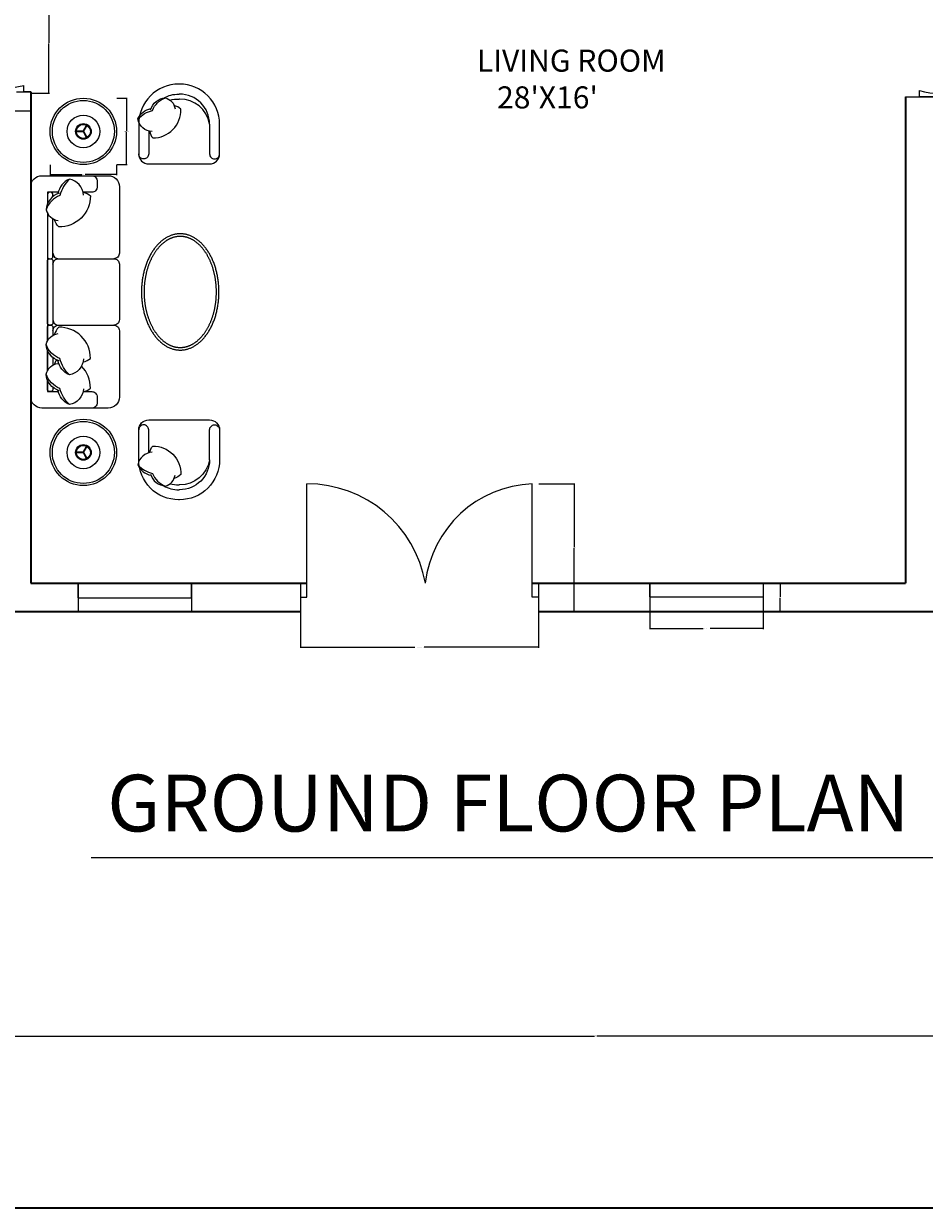
# Model space of a CAD drawing. Units: inches. Extents: x 2185 to 4426, y 1138 to 3073.
# Tile 2 of 14: x 2548 to 2834, y 1138 to 1514. Entities that reach past the tile are written whole.
import ezdxf

# ---------------------------------------------------------------- set-up
doc = ezdxf.new("R2010")
doc.units = ezdxf.units.IN
for name, color, linetype, lineweight in [('A-ANNO-DIMS', 2, 'Continuous', 18), ('A-ANNO-TITL', 7, 'Continuous', 25), ('A-ANNO-TTLB', 7, 'Continuous', 35), ('A-AREA-IDEN', 7, 'Continuous', 18), ('A-DOOR', 3, 'Continuous', 18), ('A-FURN', 8, 'Continuous', 18), ('A-GLAZ', 4, 'Continuous', 18), ('A-WALL', 7, 'Continuous', 35)]:
    doc.layers.add(name, color=color, linetype=linetype, lineweight=lineweight)
doc.styles.get("Standard").update_dxf_attribs({"font": 'arial.ttf'})
doc.dimstyles.get("Standard").update_dxf_attribs({"dimtxt": 0.18, "dimasz": 0.18, "dimexe": 0.18, "dimexo": 0.0625, "dimgap": 0.09, "dimtad": 0, "dimtih": 1, "dimtoh": 1, "dimdec": 4, "dimzin": 0, "dimdsep": 46, "dimtxsty": 'Standard', "dimcen": 0.09, "dimadec": 0, "dimazin": 0, "dimtfac": 1, "dimtdec": 4, "dimtofl": 0, "dimtmove": 0, "dimatfit": 3, "dimfxl": 1, "dimtolj": 1, "dimtzin": 0, "dimarcsym": 0})

# ---------------------------------------------------------------- blocks, each defined once
blk = doc.blocks.new('LIVING-TABLE-LAMP')
at = {"ltscale": 0.03}
for p, q in [((10.44, 10.59), (11.68, 12.74)), ((10.63, 10.48), (11.87, 12.63)), ((10.54, 10.65), (8.06, 10.65)), ((10.54, 10.43), (8.06, 10.43)), ((10.44, 10.48), (11.68, 8.34)), ((10.63, 10.59), (11.87, 8.45))]:
    blk.add_line(p, q, dxfattribs=at)
for radius in [10.54, 5.18, 2.48, 2.22]:
    blk.add_circle((10.54, 10.54), radius, dxfattribs=at)
blk.add_circle((10.54, 10.54), 9.84)
blk = doc.blocks.new('DOOR-SGL-36-BED-SW')
for p, q in [((38.25, 31.13), (33.75, 31.13)), ((33.75, 31.13), (36, 31.13)), ((36, 31.13), (36, 29.13)), ((36, 29.13), (0, 29.13)), ((36, 0), (36, 2)), ((33.75, 0), (38.25, 0)), ((38.25, 0), (36, 0))]:
    blk.add_line(p, q)
blk.add_arc((28.22, 29.13), 28.22, 180, 285.9925)
blk = doc.blocks.new('DOOR-PAIR-36-ENTRY')
for p, q in [((2, 4.5), (2, 40.5)), ((73.51, 4.5), (73.51, 40.5)), ((0, 9), (0, 0)), ((75.51, 9), (75.51, 0)), ((0, 4.5), (2, 4.5)), ((75.51, 4.5), (73.51, 4.5))]:
    blk.add_line(p, q)
for centre, radius, start, end in [((2, 2.35), 38.15, 10.036, 90), ((74.89, 4.97), 35.56, 92.226, 173.4897)]:
    blk.add_arc(centre, radius, start, end)
blk = doc.blocks.new('DOOR-SGL-36-BED-S')
for p, q in [((0, 31.73), (9, 31.73)), ((9, 31.73), (4.5, 31.73)), ((4.5, 31.73), (4.5, 31.73)), ((4.5, 31.73), (4.5, 29.73)), ((4.5, 29.73), (40.5, 29.73)), ((0, 0), (9, 0)), ((4.5, 0), (4.5, 2)), ((9, 0), (4.5, 0))]:
    blk.add_line(p, q)
blk.add_arc((11.82, 29.73), 28.68, 255.2109, 0)
blk = doc.blocks.new('WIN-PLAN-36IN-04')
for p, q in [((0, 4.34), (0, 9)), ((0, 9), (0, 0)), ((36, 4.34), (36, 9)), ((36, 9), (36, 9)), ((36, 9), (36, 0)), ((0, 4.34), (36, 4.34))]:
    blk.add_line(p, q)
blk = doc.blocks.new('WIN-PLAN-36IN-05')
for p, q in [((0, 4.66), (0, 9)), ((0, 9), (0, 0)), ((36, 9), (36, 0)), ((0, 4.66), (0, 4.66)), ((0, 4.66), (36, 4.66)), ((0, 4.66), (0, 4.66))]:
    blk.add_line(p, q)
blk = doc.blocks.new('*D52')
at = {"layer": 'A-ANNO-DIMS', "color": 0, "lineweight": -2, "transparency": 16777216}
for p, q in [((2577.3, 1490.23), (2580.58, 1490.23)), ((2580.4, 1490.05), (2580.4, 1479.87)), ((2580.4, 1469.34), (2580.4, 1479.51)), ((2577.3, 1469.16), (2580.58, 1469.16))]:
    blk.add_line(p, q, dxfattribs=at)
at = {"layer": 'A-ANNO-DIMS', "color": 0, "transparency": 16777216}
for points in [[(2580.37, 1490.05), (2580.43, 1490.05), (2580.4, 1490.23)], [(2580.37, 1469.34), (2580.43, 1469.34), (2580.4, 1469.16)]]:
    blk.add_solid(points, dxfattribs=at)
at = {"layer": 'Defpoints', "color": 0, "transparency": 16777216}
for p in [(2577.24, 1490.23), (2580.4, 1490.23), (2577.24, 1469.16)]:
    blk.add_point(p, dxfattribs=at)
at = {"layer": 'A-ANNO-DIMS', "color": 0, "transparency": 16777216, "insert": (2580.4, 1479.69), "char_height": 0.18, "attachment_point": 5}
blk.add_mtext('\\A1;LAMP 21 TYP.', dxfattribs=at)
blk = doc.blocks.new('*D53')
at = {"layer": 'A-ANNO-DIMS', "color": 0, "lineweight": -2, "transparency": 16777216}
for p, q in [((2556.17, 1469.09), (2556.17, 1465.81)), ((2556.35, 1465.99), (2566.17, 1465.99)), ((2577.06, 1465.99), (2567.23, 1465.99)), ((2577.24, 1469.09), (2577.24, 1465.81))]:
    blk.add_line(p, q, dxfattribs=at)
at = {"layer": 'A-ANNO-DIMS', "color": 0, "transparency": 16777216}
for points in [[(2556.35, 1466.02), (2556.35, 1465.96), (2556.17, 1465.99)], [(2577.06, 1466.02), (2577.06, 1465.96), (2577.24, 1465.99)]]:
    blk.add_solid(points, dxfattribs=at)
at = {"layer": 'Defpoints', "color": 0, "transparency": 16777216}
for p in [(2556.17, 1469.16), (2577.24, 1469.16), (2577.24, 1465.99)]:
    blk.add_point(p, dxfattribs=at)
at = {"layer": 'A-ANNO-DIMS', "color": 0, "transparency": 16777216, "insert": (2566.7, 1465.99), "char_height": 0.18, "attachment_point": 5}
blk.add_mtext('\\A1;21 TYP.', dxfattribs=at)
blk = doc.blocks.new('*D80')
at = {"layer": 'A-ANNO-DIMS', "color": 0, "lineweight": -2, "transparency": 16777216}
for p, q in [((2511.77, 1491.8), (2511.77, 1485.95)), ((2550.02, 1491.8), (2550.02, 1485.95)), ((2511.95, 1486.13), (2529.96, 1486.13)), ((2549.84, 1486.13), (2531.83, 1486.13))]:
    blk.add_line(p, q, dxfattribs=at)
at = {"layer": 'A-ANNO-DIMS', "color": 0, "transparency": 16777216}
for points in [[(2511.95, 1486.16), (2511.95, 1486.1), (2511.77, 1486.13)], [(2549.84, 1486.16), (2549.84, 1486.1), (2550.02, 1486.13)]]:
    blk.add_solid(points, dxfattribs=at)
at = {"layer": 'Defpoints', "color": 0, "transparency": 16777216}
for p in [(2511.77, 1491.87), (2550.02, 1491.87), (2550.02, 1486.13)]:
    blk.add_point(p, dxfattribs=at)
at = {"layer": 'A-ANNO-DIMS', "color": 0, "transparency": 16777216, "insert": (2530.89, 1486.13), "char_height": 0.18, "attachment_point": 5}
blk.add_mtext('\\A1;DOOR 38 TYP.', dxfattribs=at)
blk = doc.blocks.new('*D81')
at = {"layer": 'A-ANNO-DIMS', "color": 0, "lineweight": -2, "transparency": 16777216}
for p, q in [((2550.08, 1523.44), (2555.94, 1523.44)), ((2555.76, 1523.26), (2555.76, 1507.83)), ((2555.76, 1492.05), (2555.76, 1507.47)), ((2550.08, 1491.87), (2555.94, 1491.87))]:
    blk.add_line(p, q, dxfattribs=at)
at = {"layer": 'A-ANNO-DIMS', "color": 0, "transparency": 16777216}
for points in [[(2555.73, 1523.26), (2555.79, 1523.26), (2555.76, 1523.44)], [(2555.73, 1492.05), (2555.79, 1492.05), (2555.76, 1491.87)]]:
    blk.add_solid(points, dxfattribs=at)
at = {"layer": 'Defpoints', "color": 0, "transparency": 16777216}
for p in [(2550.02, 1523.44), (2555.76, 1523.44), (2550.02, 1491.87)]:
    blk.add_point(p, dxfattribs=at)
at = {"layer": 'A-ANNO-DIMS', "color": 0, "transparency": 16777216, "insert": (2555.76, 1507.65), "char_height": 0.18, "attachment_point": 5}
blk.add_mtext('\\A1;32 TYP.', dxfattribs=at)
blk = doc.blocks.new('*D88')
at = {"layer": 'A-ANNO-DIMS', "color": 0, "lineweight": -2, "transparency": 16777216}
for p, q in [((2635.64, 1327.31), (2635.64, 1315.87)), ((2711.16, 1327.31), (2711.16, 1315.87)), ((2635.82, 1316.05), (2671.92, 1316.05)), ((2710.98, 1316.05), (2674.88, 1316.05))]:
    blk.add_line(p, q, dxfattribs=at)
at = {"layer": 'A-ANNO-DIMS', "color": 0, "transparency": 16777216}
for points in [[(2635.82, 1316.08), (2635.82, 1316.02), (2635.64, 1316.05)], [(2710.98, 1316.08), (2710.98, 1316.02), (2711.16, 1316.05)]]:
    blk.add_solid(points, dxfattribs=at)
at = {"layer": 'Defpoints', "color": 0, "transparency": 16777216}
for p in [(2635.64, 1327.38), (2711.16, 1327.38), (2711.16, 1316.05)]:
    blk.add_point(p, dxfattribs=at)
at = {"layer": 'A-ANNO-DIMS', "color": 0, "transparency": 16777216, "insert": (2673.4, 1316.05), "char_height": 0.18, "attachment_point": 5}
blk.add_mtext('\\A1;ENTRY DOORS 76 TYP.', dxfattribs=at)
blk = doc.blocks.new('*D89')
at = {"layer": 'A-ANNO-DIMS', "color": 0, "lineweight": -2, "transparency": 16777216}
for p, q in [((2711.22, 1367.88), (2722.66, 1367.88)), ((2722.48, 1367.7), (2722.48, 1347.81)), ((2722.48, 1327.56), (2722.48, 1347.45)), ((2711.22, 1327.38), (2722.66, 1327.38))]:
    blk.add_line(p, q, dxfattribs=at)
at = {"layer": 'A-ANNO-DIMS', "color": 0, "transparency": 16777216}
for points in [[(2722.45, 1367.7), (2722.51, 1367.7), (2722.48, 1367.88)], [(2722.45, 1327.56), (2722.51, 1327.56), (2722.48, 1327.38)]]:
    blk.add_solid(points, dxfattribs=at)
at = {"layer": 'Defpoints', "color": 0, "transparency": 16777216}
for p in [(2711.16, 1367.88), (2722.48, 1367.88), (2711.16, 1327.38)]:
    blk.add_point(p, dxfattribs=at)
at = {"layer": 'A-ANNO-DIMS', "color": 0, "transparency": 16777216, "insert": (2722.48, 1347.63), "char_height": 0.18, "attachment_point": 5}
blk.add_mtext('\\A1;41 TYP.', dxfattribs=at)
blk = doc.blocks.new('*D100')
at = {"layer": 'A-ANNO-DIMS', "color": 0, "lineweight": -2, "transparency": 16777216}
for p, q in [((2746.43, 1327.31), (2746.43, 1321.8)), ((2782.43, 1327.31), (2782.43, 1321.8)), ((2746.61, 1321.98), (2763.31, 1321.98)), ((2782.25, 1321.98), (2765.55, 1321.98))]:
    blk.add_line(p, q, dxfattribs=at)
at = {"layer": 'A-ANNO-DIMS', "color": 0, "transparency": 16777216}
for points in [[(2746.61, 1322.01), (2746.61, 1321.95), (2746.43, 1321.98)], [(2782.25, 1322.01), (2782.25, 1321.95), (2782.43, 1321.98)]]:
    blk.add_solid(points, dxfattribs=at)
at = {"layer": 'Defpoints', "color": 0, "transparency": 16777216}
for p in [(2746.43, 1327.38), (2782.43, 1327.38), (2782.43, 1321.98)]:
    blk.add_point(p, dxfattribs=at)
at = {"layer": 'A-ANNO-DIMS', "color": 0, "transparency": 16777216, "insert": (2764.43, 1321.98), "char_height": 0.18, "attachment_point": 5}
blk.add_mtext('\\A1;WINDOW 36 TYP.', dxfattribs=at)
blk = doc.blocks.new('*D101')
at = {"layer": 'A-ANNO-DIMS', "color": 0, "lineweight": -2, "transparency": 16777216}
for p, q in [((2782.49, 1336.38), (2788.01, 1336.38)), ((2787.83, 1336.2), (2787.83, 1332.06)), ((2787.83, 1327.56), (2787.83, 1331.7)), ((2782.49, 1327.38), (2788.01, 1327.38))]:
    blk.add_line(p, q, dxfattribs=at)
at = {"layer": 'A-ANNO-DIMS', "color": 0, "transparency": 16777216}
for points in [[(2787.8, 1336.2), (2787.86, 1336.2), (2787.83, 1336.38)], [(2787.8, 1327.56), (2787.86, 1327.56), (2787.83, 1327.38)]]:
    blk.add_solid(points, dxfattribs=at)
at = {"layer": 'Defpoints', "color": 0, "transparency": 16777216}
for p in [(2782.43, 1336.38), (2787.83, 1336.38), (2782.43, 1327.38)]:
    blk.add_point(p, dxfattribs=at)
at = {"layer": 'A-ANNO-DIMS', "color": 0, "transparency": 16777216, "insert": (2787.83, 1331.88), "char_height": 0.18, "attachment_point": 5}
blk.add_mtext('\\A1;9 TYP.', dxfattribs=at)
blk = doc.blocks.new('*D138')
at = {"layer": 'A-ANNO-DIMS', "color": 0, "lineweight": -2, "transparency": 16777216}
for p, q in [((2368.52, 1327.31), (2368.52, 1192.47)), ((3090.02, 1327.31), (3090.02, 1192.47)), ((2368.7, 1192.65), (2728.88, 1192.65)), ((3089.84, 1192.65), (2729.66, 1192.65))]:
    blk.add_line(p, q, dxfattribs=at)
at = {"layer": 'A-ANNO-DIMS', "color": 0, "transparency": 16777216}
for points in [[(2368.7, 1192.68), (2368.7, 1192.62), (2368.52, 1192.65)], [(3089.84, 1192.68), (3089.84, 1192.62), (3090.02, 1192.65)]]:
    blk.add_solid(points, dxfattribs=at)
at = {"layer": 'Defpoints', "color": 0, "transparency": 16777216}
for p in [(2368.52, 1327.38), (3090.02, 1327.38), (3090.02, 1192.65)]:
    blk.add_point(p, dxfattribs=at)
at = {"layer": 'A-ANNO-DIMS', "color": 0, "transparency": 16777216, "insert": (2729.27, 1192.65), "char_height": 0.18, "attachment_point": 5}
blk.add_mtext('\\A1;721.5', dxfattribs=at)

msp = doc.modelspace()

# ---------------------------------------------------------------- linework, layer by layer
at = {"layer": 'A-ANNO-TITL'}
msp.add_line((2861.353, 1249.148), (2569.203, 1249.148), dxfattribs=at)
at = {"layer": 'A-ANNO-TTLB'}
msp.add_lwpolyline([(2184.741, 3073.364), (4426.252, 3073.364), (4426.252, 1137.99), (2184.741, 1137.99)], close=True, dxfattribs=at)
at = {"layer": 'A-FURN', "ltscale": 0.03}
for points in [[(2597.088, 1469.368), (2606.747, 1469.368, 0.4142136), (2609.914, 1472.535), (2609.914, 1482.036, 0.4142136), (2597.246, 1494.705), (2597.088, 1494.705), (2596.929, 1494.705, 0.4142136), (2584.261, 1482.036), (2584.261, 1472.535, 0.4142136), (2587.428, 1469.368), (2597.088, 1469.368)], [(2597.088, 1388.153), (2606.747, 1388.153, -0.4142136), (2609.914, 1384.986), (2609.914, 1375.485, -0.4142136), (2597.246, 1362.817), (2597.088, 1362.817), (2596.929, 1362.817, -0.4142136), (2584.261, 1375.485), (2584.261, 1384.986, -0.4142136), (2587.428, 1388.153), (2597.088, 1388.153)]]:
    msp.add_lwpolyline(points, format="xyb", dxfattribs=at)
at = {"layer": 'A-FURN'}
for points in [[(2584.002, 1483.635, -0.1477299), (2588.63, 1486.356, -0.2133428), (2592.714, 1490.348, -0.1786618)], [(2587.991, 1486.573, -0.3066635), (2592.714, 1490.348, -0.30633), (2595.799, 1486.901, 0.8728472)], [(2592.213, 1490.284, -0.1305915), (2596.929, 1491.538), (2597.088, 1491.538)], [(2594.23, 1489.613, -0.0723842), (2596.929, 1489.954), (2597.088, 1489.954)], [(2606.747, 1482.036, 0.4142136), (2597.246, 1491.538), (2597.088, 1491.538)], [(2606.747, 1482.036, 0.3727189), (2597.246, 1489.954), (2597.088, 1489.954)], [(2588.54, 1479.643, -0.3567724), (2584.002, 1483.635, -0.2495421), (2588.113, 1486.924, 9.6168803)], [(2587.741, 1479.74, 0.1655406), (2588.721, 1477.648, 0.4259892), (2597.614, 1486.719, 0.1215233), (2595.503, 1487.97, -7.1154643)], [(2606.747, 1482.037), (2606.747, 1472.535, 0.4142136), (2608.331, 1470.952), (2608.331, 1470.952, 0.4142136), (2609.914, 1472.535)], [(2587.428, 1479.816), (2587.428, 1472.535, -0.4142136), (2585.845, 1470.952), (2585.845, 1470.952, -0.4142136), (2584.261, 1472.535)], [(2562.297, 1464.525, 0.1477299), (2559.278, 1459.392, 0.2133428), (2554.851, 1454.862, 0.1786618)], [(2566.724, 1459.492, 0.3567724), (2562.297, 1464.525, 0.2495421), (2558.649, 1459.965, -9.6168803)], [(2569.338, 1465.643, -0.4142136), (2571.095, 1463.886), (2571.095, 1462.13, -0.4142136), (2569.338, 1460.374), (2566.617, 1460.374)], [(2559.038, 1460.101, 0.3066635), (2554.851, 1454.862, 0.30633), (2558.675, 1451.44, -0.8728472)], [(2557.044, 1459.033), (2557.044, 1459.671, 0.4142136), (2556.342, 1460.374), (2555.991, 1460.374, 0.4142136), (2555.288, 1459.671)], [(2555.288, 1459.671), (2555.288, 1456.679, 0.4142136)], [(2566.617, 1460.378, -0.1655406), (2568.937, 1459.291, -0.4259892), (2558.876, 1449.427, -0.1215233), (2557.489, 1451.769, 7.1154643)], [(2555.288, 1453.757), (2555.288, 1440.001, 0.4142136), (2555.991, 1439.298), (2556.342, 1439.298, 0.4142136), (2557.044, 1440.001), (2557.044, 1451.989, 0.4142136)], [(2557.044, 1441.055, 0.4142136), (2558.801, 1439.298), (2576.364, 1439.298, 0.4142136)], [(2557.044, 1437.542, -0.4142136), (2558.801, 1439.298)], [(2555.288, 1413.225), (2555.288, 1417.52, -0.4142136), (2555.991, 1418.223), (2556.342, 1418.223, -0.4142136), (2557.044, 1417.52), (2557.044, 1414.994, -0.4142136)], [(2557.044, 1419.979, 0.4142136), (2558.801, 1418.223)], [(2557.044, 1416.467, -0.4142136), (2558.801, 1418.223), (2576.364, 1418.223, -0.4142136)], [(2566.617, 1406.605, 0.1655406), (2568.937, 1407.691, 0.4259892), (2558.876, 1417.555, 0.1215233), (2557.489, 1415.213, -7.1154643)], [(2559.038, 1406.881, -0.3066635), (2554.851, 1412.12, -0.30633), (2558.675, 1415.542, 0.8728472)], [(2562.297, 1402.457, -0.1477299), (2559.278, 1407.591, -0.2133428), (2554.851, 1412.12, -0.1786618)], [(2555.288, 1403.764), (2555.288, 1410.303, -0.4142136)], [(2559.038, 1397.42, -0.3066635), (2554.851, 1402.659, -0.30633), (2558.675, 1406.081, 0.8728472)], [(2557.044, 1407.949), (2557.044, 1405.532, -0.4142136)], [(2558.176, 1407.225, 0.0718654), (2557.489, 1405.752, -7.1154643)], [(2566.724, 1407.49, -0.3567724), (2562.297, 1402.457, -0.2495421), (2558.649, 1407.017, 9.6168803)], [(2562.297, 1392.996, -0.1477299), (2559.278, 1398.129, -0.2133428), (2554.851, 1402.659, -0.1786618)], [(2566.617, 1397.144, 0.1655406), (2568.937, 1398.23, 0.2002311), (2566.111, 1405.202, 0.1215233)], [(2555.288, 1400.842), (2555.288, 1397.147), (2558.74, 1397.147, -0.4142136)], [(2555.288, 1397.85), (2555.288, 1400.842, -0.4142136)], [(2557.044, 1398.488), (2557.044, 1397.85, -0.4142136), (2556.342, 1397.147), (2555.991, 1397.147, -0.4142136), (2555.288, 1397.85)], [(2566.724, 1398.029, -0.3567724), (2562.297, 1392.996, -0.2495421), (2558.649, 1397.556, 9.6168803)], [(2566.617, 1397.147), (2569.338, 1397.147, -0.4142136), (2571.095, 1395.391), (2571.095, 1393.635, -0.4142136), (2569.338, 1391.879)], [(2587.428, 1377.705), (2587.428, 1384.986, 0.4142136), (2585.845, 1386.57), (2585.845, 1386.57, 0.4142136), (2584.261, 1384.986)], [(2606.747, 1375.485), (2606.747, 1384.986, -0.4142136), (2608.331, 1386.57), (2608.331, 1386.57, -0.4142136), (2609.914, 1384.986)], [(2587.741, 1377.781, -0.1655406), (2588.721, 1379.873, -0.4259892), (2597.614, 1370.802, -0.1215233), (2595.503, 1369.552, 7.1154643)], [(2588.54, 1377.878, 0.3567724), (2584.002, 1373.886, 0.2495421), (2588.113, 1370.597, -9.6168803)], [(2584.002, 1373.886, 0.1477299), (2588.63, 1371.165, 0.2133428), (2592.714, 1367.173, 0.1786618)], [(2606.747, 1375.485, -0.3727189), (2597.246, 1367.567), (2597.088, 1367.567)], [(2606.747, 1375.485, -0.4142136), (2597.246, 1365.984), (2597.088, 1365.984)], [(2587.991, 1370.948, 0.3066635), (2592.714, 1367.173, 0.30633), (2595.799, 1370.621, -0.8728472)], [(2592.213, 1367.237, 0.1305915), (2596.929, 1365.984), (2597.088, 1365.984)], [(2594.23, 1367.908, 0.0723842), (2596.929, 1367.567), (2597.088, 1367.567)]]:
    msp.add_lwpolyline(points, format="xyb", dxfattribs=at)
at = {"layer": 'A-FURN', "ltscale": 0.03}
msp.add_lwpolyline([(2574.607, 1465.643, -0.4142136), (2578.12, 1462.13), (2578.12, 1441.055, -0.4142136), (2576.364, 1439.298, -0.4142136), (2578.12, 1437.542), (2578.12, 1419.979, -0.4142136), (2576.364, 1418.223, -0.4142136), (2578.12, 1416.467), (2578.12, 1395.391, -0.4142136), (2574.607, 1391.879), (2553.532, 1391.879, -0.4142136), (2550.019, 1395.391), (2550.019, 1462.13, -0.4142136), (2553.532, 1465.643)], format="xyb", close=True, dxfattribs=at)
at = {"layer": 'A-FURN'}
for points in [[(2558.74, 1460.374), (2555.288, 1460.374), (2555.288, 1456.679)], [(2555.288, 1453.757), (2555.288, 1413.225)], [(2555.288, 1410.303), (2555.288, 1403.764)]]:
    msp.add_lwpolyline(points, dxfattribs=at)
msp.add_lwpolyline([(2555.288, 1418.925), (2555.288, 1438.596, -0.4142136), (2555.991, 1439.298), (2556.342, 1439.298, -0.4142136), (2557.044, 1438.596), (2557.044, 1418.925, -0.4142136), (2556.342, 1418.223), (2555.991, 1418.223, -0.4142136)], format="xyb", close=True, dxfattribs=at)
at = {"layer": 'A-FURN', "ltscale": 0.03}
msp.add_polyline3d([(2597.439, 1447.202, 0), (2597.206, 1447.198, 0), (2596.974, 1447.188, 0), (2596.741, 1447.172, 0), (2596.509, 1447.149, 0), (2596.277, 1447.119, 0), (2596.046, 1447.083, 0), (2595.815, 1447.04, 0), (2595.585, 1446.991, 0), (2595.355, 1446.935, 0), (2595.126, 1446.872, 0), (2594.898, 1446.803, 0), (2594.671, 1446.728, 0), (2594.445, 1446.646, 0), (2594.22, 1446.558, 0), (2593.996, 1446.463, 0), (2593.773, 1446.363, 0), (2593.552, 1446.255, 0), (2593.331, 1446.142, 0), (2593.113, 1446.022, 0), (2592.896, 1445.896, 0), (2592.681, 1445.764, 0), (2592.467, 1445.626, 0), (2592.255, 1445.482, 0), (2592.045, 1445.332, 0), (2591.837, 1445.176, 0), (2591.631, 1445.014, 0), (2591.427, 1444.846, 0), (2591.225, 1444.672, 0), (2591.025, 1444.493, 0), (2590.828, 1444.308, 0), (2590.633, 1444.118, 0), (2590.44, 1443.922, 0), (2590.25, 1443.721, 0), (2590.063, 1443.514, 0), (2589.878, 1443.302, 0), (2589.696, 1443.085, 0), (2589.517, 1442.862, 0), (2589.34, 1442.635, 0), (2589.167, 1442.402, 0), (2588.996, 1442.165, 0), (2588.828, 1441.923, 0), (2588.664, 1441.676, 0), (2588.503, 1441.425, 0), (2588.344, 1441.169, 0), (2588.189, 1440.909, 0), (2588.038, 1440.644, 0), (2587.89, 1440.375, 0), (2587.745, 1440.102, 0), (2587.603, 1439.825, 0), (2587.466, 1439.543, 0), (2587.331, 1439.258, 0), (2587.201, 1438.97, 0), (2587.074, 1438.677, 0), (2586.951, 1438.381, 0), (2586.831, 1438.082, 0), (2586.715, 1437.779, 0), (2586.604, 1437.473, 0), (2586.496, 1437.164, 0), (2586.391, 1436.852, 0), (2586.291, 1436.536, 0), (2586.195, 1436.219, 0), (2586.103, 1435.898, 0), (2586.015, 1435.575, 0), (2585.931, 1435.25, 0), (2585.851, 1434.922, 0), (2585.776, 1434.592, 0), (2585.704, 1434.26, 0), (2585.637, 1433.926, 0), (2585.574, 1433.59, 0), (2585.515, 1433.252, 0), (2585.461, 1432.913, 0), (2585.41, 1432.572, 0), (2585.364, 1432.23, 0), (2585.323, 1431.886, 0), (2585.286, 1431.542, 0), (2585.253, 1431.196, 0), (2585.224, 1430.85, 0), (2585.2, 1430.503, 0), (2585.18, 1430.155, 0), (2585.165, 1429.807, 0), (2585.154, 1429.458, 0), (2585.147, 1429.11, 0), (2585.145, 1428.761, 0), (2585.147, 1428.412, 0), (2585.154, 1428.063, 0), (2585.165, 1427.714, 0), (2585.18, 1427.366, 0), (2585.2, 1427.018, 0), (2585.224, 1426.671, 0), (2585.253, 1426.325, 0), (2585.286, 1425.979, 0), (2585.323, 1425.635, 0), (2585.364, 1425.291, 0), (2585.41, 1424.949, 0), (2585.461, 1424.608, 0), (2585.515, 1424.269, 0), (2585.574, 1423.932, 0), (2585.637, 1423.596, 0), (2585.704, 1423.262, 0), (2585.776, 1422.929, 0), (2585.851, 1422.599, 0), (2585.931, 1422.272, 0), (2586.015, 1421.946, 0), (2586.103, 1421.623, 0), (2586.195, 1421.302, 0), (2586.291, 1420.985, 0), (2586.391, 1420.67, 0), (2586.496, 1420.357, 0), (2586.604, 1420.048, 0), (2586.715, 1419.742, 0), (2586.831, 1419.44, 0), (2586.951, 1419.14, 0), (2587.074, 1418.844, 0), (2587.201, 1418.552, 0), (2587.331, 1418.263, 0), (2587.466, 1417.978, 0), (2587.603, 1417.697, 0), (2587.745, 1417.419, 0), (2587.89, 1417.146, 0), (2588.038, 1416.877, 0), (2588.189, 1416.613, 0), (2588.344, 1416.352, 0), (2588.503, 1416.096, 0), (2588.664, 1415.845, 0), (2588.828, 1415.598, 0), (2588.996, 1415.356, 0), (2589.167, 1415.119, 0), (2589.34, 1414.886, 0), (2589.517, 1414.659, 0), (2589.696, 1414.437, 0), (2589.878, 1414.219, 0), (2590.063, 1414.007, 0), (2590.25, 1413.801, 0), (2590.44, 1413.599, 0), (2590.633, 1413.403, 0), (2590.828, 1413.213, 0), (2591.025, 1413.028, 0), (2591.225, 1412.849, 0), (2591.427, 1412.675, 0), (2591.631, 1412.507, 0), (2591.837, 1412.345, 0), (2592.045, 1412.189, 0), (2592.255, 1412.039, 0), (2592.467, 1411.895, 0), (2592.681, 1411.757, 0), (2592.896, 1411.625, 0), (2593.113, 1411.499, 0), (2593.331, 1411.379, 0), (2593.552, 1411.266, 0), (2593.773, 1411.159, 0), (2593.996, 1411.058, 0), (2594.22, 1410.963, 0), (2594.445, 1410.875, 0), (2594.671, 1410.793, 0), (2594.898, 1410.718, 0), (2595.126, 1410.649, 0), (2595.355, 1410.586, 0), (2595.585, 1410.531, 0), (2595.815, 1410.481, 0), (2596.046, 1410.438, 0), (2596.277, 1410.402, 0), (2596.509, 1410.372, 0), (2596.741, 1410.349, 0), (2596.974, 1410.333, 0), (2597.206, 1410.323, 0), (2597.439, 1410.32, 0), (2597.672, 1410.323, 0), (2597.904, 1410.333, 0), (2598.137, 1410.349, 0), (2598.369, 1410.372, 0), (2598.601, 1410.402, 0), (2598.832, 1410.438, 0), (2599.063, 1410.481, 0), (2599.293, 1410.531, 0), (2599.523, 1410.586, 0), (2599.752, 1410.649, 0), (2599.98, 1410.718, 0), (2600.207, 1410.793, 0), (2600.433, 1410.875, 0), (2600.658, 1410.963, 0), (2600.882, 1411.058, 0), (2601.105, 1411.159, 0), (2601.326, 1411.266, 0), (2601.546, 1411.379, 0), (2601.765, 1411.499, 0), (2601.982, 1411.625, 0), (2602.197, 1411.757, 0), (2602.411, 1411.895, 0), (2602.623, 1412.039, 0), (2602.833, 1412.189, 0), (2603.041, 1412.345, 0), (2603.247, 1412.507, 0), (2603.451, 1412.675, 0), (2603.653, 1412.849, 0), (2603.853, 1413.028, 0), (2604.05, 1413.213, 0), (2604.245, 1413.403, 0), (2604.437, 1413.599, 0), (2604.627, 1413.801, 0), (2604.815, 1414.007, 0), (2605, 1414.219, 0), (2605.182, 1414.437, 0), (2605.361, 1414.659, 0), (2605.538, 1414.886, 0), (2605.711, 1415.119, 0), (2605.882, 1415.356, 0), (2606.049, 1415.598, 0), (2606.214, 1415.845, 0), (2606.375, 1416.096, 0), (2606.534, 1416.352, 0), (2606.688, 1416.613, 0), (2606.84, 1416.877, 0), (2606.988, 1417.146, 0), (2607.133, 1417.419, 0), (2607.274, 1417.697, 0), (2607.412, 1417.978, 0), (2607.547, 1418.263, 0), (2607.677, 1418.552, 0), (2607.804, 1418.844, 0), (2607.927, 1419.14, 0), (2608.047, 1419.44, 0), (2608.163, 1419.742, 0), (2608.274, 1420.048, 0), (2608.382, 1420.357, 0), (2608.486, 1420.67, 0), (2608.587, 1420.985, 0), (2608.683, 1421.302, 0), (2608.775, 1421.623, 0), (2608.863, 1421.946, 0), (2608.947, 1422.272, 0), (2609.027, 1422.599, 0), (2609.102, 1422.929, 0), (2609.174, 1423.262, 0), (2609.241, 1423.596, 0), (2609.304, 1423.932, 0), (2609.363, 1424.269, 0), (2609.417, 1424.608, 0), (2609.468, 1424.949, 0), (2609.513, 1425.291, 0), (2609.555, 1425.635, 0), (2609.592, 1425.979, 0), (2609.625, 1426.325, 0), (2609.654, 1426.671, 0), (2609.678, 1427.018, 0), (2609.698, 1427.366, 0), (2609.713, 1427.714, 0), (2609.724, 1428.063, 0), (2609.731, 1428.412, 0), (2609.733, 1428.761, 0), (2609.731, 1429.11, 0), (2609.724, 1429.458, 0), (2609.713, 1429.807, 0), (2609.698, 1430.155, 0), (2609.678, 1430.503, 0), (2609.654, 1430.85, 0), (2609.625, 1431.196, 0), (2609.592, 1431.542, 0), (2609.555, 1431.886, 0), (2609.513, 1432.23, 0), (2609.468, 1432.572, 0), (2609.417, 1432.913, 0), (2609.363, 1433.252, 0), (2609.304, 1433.59, 0), (2609.241, 1433.926, 0), (2609.174, 1434.26, 0), (2609.102, 1434.592, 0), (2609.027, 1434.922, 0), (2608.947, 1435.25, 0), (2608.863, 1435.575, 0), (2608.775, 1435.898, 0), (2608.683, 1436.219, 0), (2608.587, 1436.536, 0), (2608.486, 1436.852, 0), (2608.382, 1437.164, 0), (2608.274, 1437.473, 0), (2608.163, 1437.779, 0), (2608.047, 1438.082, 0), (2607.927, 1438.381, 0), (2607.804, 1438.677, 0), (2607.677, 1438.97, 0), (2607.547, 1439.258, 0), (2607.412, 1439.543, 0), (2607.274, 1439.825, 0), (2607.133, 1440.102, 0), (2606.988, 1440.375, 0), (2606.84, 1440.644, 0), (2606.688, 1440.909, 0), (2606.534, 1441.169, 0), (2606.375, 1441.425, 0), (2606.214, 1441.676, 0), (2606.049, 1441.923, 0), (2605.882, 1442.165, 0), (2605.711, 1442.402, 0), (2605.538, 1442.635, 0), (2605.361, 1442.862, 0), (2605.182, 1443.085, 0), (2605, 1443.302, 0), (2604.815, 1443.514, 0), (2604.627, 1443.721, 0), (2604.437, 1443.922, 0), (2604.245, 1444.118, 0), (2604.05, 1444.308, 0), (2603.853, 1444.493, 0), (2603.653, 1444.672, 0), (2603.451, 1444.846, 0), (2603.247, 1445.014, 0), (2603.041, 1445.176, 0), (2602.833, 1445.332, 0), (2602.623, 1445.482, 0), (2602.411, 1445.626, 0), (2602.197, 1445.764, 0), (2601.982, 1445.896, 0), (2601.765, 1446.022, 0), (2601.546, 1446.142, 0), (2601.326, 1446.255, 0), (2601.105, 1446.363, 0), (2600.882, 1446.463, 0), (2600.658, 1446.558, 0), (2600.433, 1446.646, 0), (2600.207, 1446.728, 0), (2599.98, 1446.803, 0), (2599.752, 1446.872, 0), (2599.523, 1446.935, 0), (2599.293, 1446.991, 0), (2599.063, 1447.04, 0), (2598.832, 1447.083, 0), (2598.601, 1447.119, 0), (2598.369, 1447.149, 0), (2598.137, 1447.172, 0), (2597.904, 1447.188, 0), (2597.672, 1447.198, 0), (2597.439, 1447.202, 0)], dxfattribs=at)
at = {"layer": 'A-FURN'}
msp.add_polyline3d([(2597.439, 1446.382, 0), (2597.313, 1446.381, 0), (2597.187, 1446.378, 0), (2597.06, 1446.372, 0), (2596.933, 1446.365, 0), (2596.805, 1446.355, 0), (2596.676, 1446.342, 0), (2596.547, 1446.328, 0), (2596.418, 1446.311, 0), (2596.288, 1446.292, 0), (2596.158, 1446.27, 0), (2596.027, 1446.246, 0), (2595.896, 1446.22, 0), (2595.764, 1446.191, 0), (2595.632, 1446.159, 0), (2595.5, 1446.125, 0), (2595.367, 1446.089, 0), (2595.235, 1446.05, 0), (2595.101, 1446.008, 0), (2594.968, 1445.963, 0), (2594.834, 1445.916, 0), (2594.7, 1445.867, 0), (2594.566, 1445.814, 0), (2594.432, 1445.759, 0), (2594.297, 1445.7, 0), (2594.162, 1445.64, 0), (2594.028, 1445.576, 0), (2593.893, 1445.509, 0), (2593.759, 1445.44, 0), (2593.624, 1445.368, 0), (2593.49, 1445.293, 0), (2593.355, 1445.215, 0), (2593.221, 1445.135, 0), (2593.087, 1445.051, 0), (2592.954, 1444.965, 0), (2592.821, 1444.876, 0), (2592.688, 1444.784, 0), (2592.555, 1444.689, 0), (2592.423, 1444.592, 0), (2592.292, 1444.491, 0), (2592.161, 1444.388, 0), (2592.03, 1444.282, 0), (2591.9, 1444.173, 0), (2591.771, 1444.061, 0), (2591.642, 1443.946, 0), (2591.514, 1443.828, 0), (2591.387, 1443.706, 0), (2591.261, 1443.582, 0), (2591.135, 1443.455, 0), (2591.01, 1443.326, 0), (2590.886, 1443.193, 0), (2590.763, 1443.058, 0), (2590.641, 1442.92, 0), (2590.52, 1442.779, 0), (2590.399, 1442.636, 0), (2590.28, 1442.49, 0), (2590.162, 1442.341, 0), (2590.045, 1442.19, 0), (2589.929, 1442.037, 0), (2589.814, 1441.881, 0), (2589.701, 1441.722, 0), (2589.588, 1441.562, 0), (2589.477, 1441.399, 0), (2589.368, 1441.234, 0), (2589.259, 1441.067, 0), (2589.152, 1440.897, 0), (2589.046, 1440.725, 0), (2588.942, 1440.552, 0), (2588.839, 1440.376, 0), (2588.738, 1440.198, 0), (2588.638, 1440.019, 0), (2588.54, 1439.837, 0), (2588.443, 1439.654, 0), (2588.348, 1439.468, 0), (2588.255, 1439.281, 0), (2588.163, 1439.093, 0), (2588.074, 1438.902, 0), (2587.985, 1438.71, 0), (2587.899, 1438.517, 0), (2587.815, 1438.321, 0), (2587.732, 1438.125, 0), (2587.651, 1437.926, 0), (2587.573, 1437.727, 0), (2587.496, 1437.526, 0), (2587.421, 1437.324, 0), (2587.348, 1437.121, 0), (2587.277, 1436.918, 0), (2587.208, 1436.714, 0), (2587.141, 1436.509, 0), (2587.076, 1436.305, 0), (2587.013, 1436.099, 0), (2586.952, 1435.893, 0), (2586.893, 1435.687, 0), (2586.836, 1435.48, 0), (2586.78, 1435.273, 0), (2586.727, 1435.066, 0), (2586.675, 1434.858, 0), (2586.626, 1434.649, 0), (2586.578, 1434.44, 0), (2586.532, 1434.231, 0), (2586.488, 1434.022, 0), (2586.446, 1433.812, 0), (2586.405, 1433.601, 0), (2586.367, 1433.391, 0), (2586.33, 1433.18, 0), (2586.295, 1432.969, 0), (2586.262, 1432.758, 0), (2586.231, 1432.546, 0), (2586.201, 1432.334, 0), (2586.173, 1432.122, 0), (2586.147, 1431.909, 0), (2586.123, 1431.697, 0), (2586.101, 1431.484, 0), (2586.08, 1431.271, 0), (2586.061, 1431.058, 0), (2586.044, 1430.845, 0), (2586.028, 1430.631, 0), (2586.014, 1430.418, 0), (2586.002, 1430.204, 0), (2585.992, 1429.991, 0), (2585.983, 1429.777, 0), (2585.976, 1429.563, 0), (2585.971, 1429.349, 0), (2585.967, 1429.135, 0), (2585.965, 1428.921, 0), (2585.965, 1428.707, 0), (2585.966, 1428.493, 0), (2585.969, 1428.279, 0), (2585.973, 1428.065, 0), (2585.979, 1427.851, 0), (2585.987, 1427.637, 0), (2585.997, 1427.424, 0), (2586.008, 1427.21, 0), (2586.021, 1426.996, 0), (2586.036, 1426.783, 0), (2586.052, 1426.57, 0), (2586.07, 1426.357, 0), (2586.09, 1426.143, 0), (2586.112, 1425.931, 0), (2586.135, 1425.718, 0), (2586.16, 1425.505, 0), (2586.187, 1425.293, 0), (2586.216, 1425.081, 0), (2586.246, 1424.869, 0), (2586.278, 1424.658, 0), (2586.312, 1424.447, 0), (2586.348, 1424.236, 0), (2586.386, 1424.025, 0), (2586.425, 1423.815, 0), (2586.467, 1423.604, 0), (2586.51, 1423.395, 0), (2586.555, 1423.185, 0), (2586.602, 1422.976, 0), (2586.65, 1422.768, 0), (2586.701, 1422.559, 0), (2586.754, 1422.352, 0), (2586.808, 1422.144, 0), (2586.864, 1421.937, 0), (2586.922, 1421.731, 0), (2586.983, 1421.525, 0), (2587.045, 1421.319, 0), (2587.109, 1421.114, 0), (2587.175, 1420.909, 0), (2587.243, 1420.705, 0), (2587.312, 1420.502, 0), (2587.384, 1420.299, 0), (2587.458, 1420.096, 0), (2587.534, 1419.895, 0), (2587.612, 1419.694, 0), (2587.691, 1419.495, 0), (2587.773, 1419.298, 0), (2587.857, 1419.102, 0), (2587.942, 1418.908, 0), (2588.029, 1418.715, 0), (2588.118, 1418.523, 0), (2588.209, 1418.334, 0), (2588.302, 1418.146, 0), (2588.396, 1417.96, 0), (2588.491, 1417.776, 0), (2588.589, 1417.593, 0), (2588.688, 1417.412, 0), (2588.788, 1417.234, 0), (2588.89, 1417.057, 0), (2588.994, 1416.882, 0), (2589.099, 1416.71, 0), (2589.205, 1416.539, 0), (2589.313, 1416.371, 0), (2589.422, 1416.204, 0), (2589.533, 1416.04, 0), (2589.644, 1415.879, 0), (2589.757, 1415.719, 0), (2589.871, 1415.562, 0), (2589.987, 1415.407, 0), (2590.103, 1415.255, 0), (2590.221, 1415.105, 0), (2590.34, 1414.958, 0), (2590.459, 1414.814, 0), (2590.58, 1414.672, 0), (2590.702, 1414.532, 0), (2590.824, 1414.395, 0), (2590.948, 1414.261, 0), (2591.072, 1414.13, 0), (2591.198, 1414.002, 0), (2591.324, 1413.876, 0), (2591.451, 1413.754, 0), (2591.578, 1413.634, 0), (2591.706, 1413.518, 0), (2591.835, 1413.404, 0), (2591.965, 1413.293, 0), (2592.095, 1413.186, 0), (2592.226, 1413.081, 0), (2592.357, 1412.979, 0), (2592.489, 1412.88, 0), (2592.622, 1412.784, 0), (2592.754, 1412.691, 0), (2592.887, 1412.6, 0), (2593.021, 1412.513, 0), (2593.154, 1412.428, 0), (2593.288, 1412.346, 0), (2593.422, 1412.267, 0), (2593.557, 1412.19, 0), (2593.691, 1412.117, 0), (2593.826, 1412.046, 0), (2593.961, 1411.978, 0), (2594.095, 1411.913, 0), (2594.23, 1411.851, 0), (2594.364, 1411.791, 0), (2594.499, 1411.735, 0), (2594.633, 1411.681, 0), (2594.767, 1411.629, 0), (2594.901, 1411.581, 0), (2595.035, 1411.535, 0), (2595.168, 1411.492, 0), (2595.301, 1411.452, 0), (2595.434, 1411.414, 0), (2595.566, 1411.378, 0), (2595.698, 1411.346, 0), (2595.83, 1411.316, 0), (2595.961, 1411.288, 0), (2596.092, 1411.263, 0), (2596.223, 1411.24, 0), (2596.353, 1411.219, 0), (2596.483, 1411.201, 0), (2596.612, 1411.186, 0), (2596.741, 1411.172, 0), (2596.869, 1411.161, 0), (2596.996, 1411.152, 0), (2597.124, 1411.146, 0), (2597.25, 1411.142, 0), (2597.376, 1411.139, 0), (2597.502, 1411.139, 0), (2597.628, 1411.142, 0), (2597.754, 1411.146, 0), (2597.882, 1411.152, 0), (2598.009, 1411.161, 0), (2598.137, 1411.172, 0), (2598.266, 1411.186, 0), (2598.395, 1411.201, 0), (2598.525, 1411.219, 0), (2598.655, 1411.24, 0), (2598.786, 1411.263, 0), (2598.917, 1411.288, 0), (2599.048, 1411.316, 0), (2599.18, 1411.346, 0), (2599.312, 1411.378, 0), (2599.444, 1411.414, 0), (2599.577, 1411.452, 0), (2599.71, 1411.492, 0), (2599.843, 1411.535, 0), (2599.977, 1411.581, 0), (2600.111, 1411.629, 0), (2600.245, 1411.681, 0), (2600.379, 1411.735, 0), (2600.514, 1411.791, 0), (2600.648, 1411.851, 0), (2600.783, 1411.913, 0), (2600.917, 1411.978, 0), (2601.052, 1412.046, 0), (2601.187, 1412.117, 0), (2601.321, 1412.19, 0), (2601.455, 1412.267, 0), (2601.59, 1412.346, 0), (2601.724, 1412.428, 0), (2601.857, 1412.513, 0), (2601.991, 1412.6, 0), (2602.124, 1412.691, 0), (2602.256, 1412.784, 0), (2602.389, 1412.88, 0), (2602.521, 1412.979, 0), (2602.652, 1413.081, 0), (2602.783, 1413.186, 0), (2602.913, 1413.293, 0), (2603.043, 1413.404, 0), (2603.171, 1413.518, 0), (2603.3, 1413.634, 0), (2603.427, 1413.754, 0), (2603.554, 1413.876, 0), (2603.68, 1414.002, 0), (2603.806, 1414.13, 0), (2603.93, 1414.261, 0), (2604.054, 1414.395, 0), (2604.176, 1414.532, 0), (2604.298, 1414.672, 0), (2604.419, 1414.814, 0), (2604.538, 1414.958, 0), (2604.657, 1415.105, 0), (2604.775, 1415.255, 0), (2604.891, 1415.407, 0), (2605.006, 1415.562, 0), (2605.121, 1415.719, 0), (2605.234, 1415.879, 0), (2605.345, 1416.04, 0), (2605.456, 1416.204, 0), (2605.565, 1416.371, 0), (2605.673, 1416.539, 0), (2605.779, 1416.71, 0), (2605.884, 1416.882, 0), (2605.987, 1417.057, 0), (2606.09, 1417.234, 0), (2606.19, 1417.412, 0), (2606.289, 1417.593, 0), (2606.386, 1417.776, 0), (2606.482, 1417.96, 0), (2606.576, 1418.146, 0), (2606.669, 1418.334, 0), (2606.76, 1418.523, 0), (2606.849, 1418.715, 0), (2606.936, 1418.908, 0), (2607.021, 1419.102, 0), (2607.105, 1419.298, 0), (2607.186, 1419.495, 0), (2607.266, 1419.694, 0), (2607.344, 1419.895, 0), (2607.42, 1420.096, 0), (2607.494, 1420.299, 0), (2607.566, 1420.502, 0), (2607.635, 1420.705, 0), (2607.703, 1420.909, 0), (2607.769, 1421.114, 0), (2607.833, 1421.319, 0), (2607.895, 1421.525, 0), (2607.955, 1421.731, 0), (2608.014, 1421.937, 0), (2608.07, 1422.144, 0), (2608.124, 1422.352, 0), (2608.177, 1422.559, 0), (2608.228, 1422.768, 0), (2608.276, 1422.976, 0), (2608.323, 1423.185, 0), (2608.368, 1423.395, 0), (2608.411, 1423.604, 0), (2608.453, 1423.815, 0), (2608.492, 1424.025, 0), (2608.53, 1424.236, 0), (2608.566, 1424.447, 0), (2608.6, 1424.658, 0), (2608.632, 1424.869, 0), (2608.662, 1425.081, 0), (2608.691, 1425.293, 0), (2608.718, 1425.505, 0), (2608.743, 1425.718, 0), (2608.766, 1425.931, 0), (2608.788, 1426.143, 0), (2608.808, 1426.357, 0), (2608.826, 1426.57, 0), (2608.842, 1426.783, 0), (2608.857, 1426.996, 0), (2608.87, 1427.21, 0), (2608.881, 1427.424, 0), (2608.891, 1427.637, 0), (2608.898, 1427.851, 0), (2608.905, 1428.065, 0), (2608.909, 1428.279, 0), (2608.912, 1428.493, 0), (2608.913, 1428.707, 0), (2608.913, 1428.921, 0), (2608.911, 1429.135, 0), (2608.907, 1429.349, 0), (2608.902, 1429.563, 0), (2608.895, 1429.777, 0), (2608.886, 1429.991, 0), (2608.876, 1430.204, 0), (2608.863, 1430.418, 0), (2608.85, 1430.631, 0), (2608.834, 1430.845, 0), (2608.817, 1431.058, 0), (2608.798, 1431.271, 0), (2608.777, 1431.484, 0), (2608.755, 1431.697, 0), (2608.731, 1431.909, 0), (2608.705, 1432.122, 0), (2608.677, 1432.334, 0), (2608.647, 1432.546, 0), (2608.616, 1432.758, 0), (2608.583, 1432.969, 0), (2608.548, 1433.18, 0), (2608.511, 1433.391, 0), (2608.473, 1433.601, 0), (2608.432, 1433.812, 0), (2608.39, 1434.022, 0), (2608.346, 1434.231, 0), (2608.3, 1434.44, 0), (2608.252, 1434.649, 0), (2608.202, 1434.858, 0), (2608.151, 1435.066, 0), (2608.097, 1435.273, 0), (2608.042, 1435.48, 0), (2607.985, 1435.687, 0), (2607.926, 1435.893, 0), (2607.865, 1436.099, 0), (2607.802, 1436.305, 0), (2607.737, 1436.509, 0), (2607.67, 1436.714, 0), (2607.601, 1436.918, 0), (2607.53, 1437.121, 0), (2607.457, 1437.324, 0), (2607.382, 1437.526, 0), (2607.305, 1437.727, 0), (2607.227, 1437.926, 0), (2607.146, 1438.125, 0), (2607.063, 1438.321, 0), (2606.979, 1438.517, 0), (2606.892, 1438.71, 0), (2606.804, 1438.902, 0), (2606.714, 1439.093, 0), (2606.623, 1439.281, 0), (2606.53, 1439.468, 0), (2606.435, 1439.654, 0), (2606.338, 1439.837, 0), (2606.24, 1440.019, 0), (2606.14, 1440.198, 0), (2606.039, 1440.376, 0), (2605.936, 1440.552, 0), (2605.832, 1440.725, 0), (2605.726, 1440.897, 0), (2605.619, 1441.067, 0), (2605.51, 1441.234, 0), (2605.401, 1441.399, 0), (2605.29, 1441.562, 0), (2605.177, 1441.722, 0), (2605.064, 1441.881, 0), (2604.949, 1442.037, 0), (2604.833, 1442.19, 0), (2604.716, 1442.341, 0), (2604.598, 1442.49, 0), (2604.479, 1442.636, 0), (2604.358, 1442.779, 0), (2604.237, 1442.92, 0), (2604.115, 1443.058, 0), (2603.992, 1443.193, 0), (2603.868, 1443.326, 0), (2603.743, 1443.455, 0), (2603.617, 1443.582, 0), (2603.491, 1443.706, 0), (2603.364, 1443.828, 0), (2603.236, 1443.946, 0), (2603.107, 1444.061, 0), (2602.978, 1444.173, 0), (2602.848, 1444.282, 0), (2602.717, 1444.388, 0), (2602.586, 1444.491, 0), (2602.455, 1444.592, 0), (2602.323, 1444.689, 0), (2602.19, 1444.784, 0), (2602.057, 1444.876, 0), (2601.924, 1444.965, 0), (2601.79, 1445.051, 0), (2601.657, 1445.135, 0), (2601.523, 1445.215, 0), (2601.388, 1445.293, 0), (2601.254, 1445.368, 0), (2601.119, 1445.44, 0), (2600.985, 1445.509, 0), (2600.85, 1445.576, 0), (2600.715, 1445.64, 0), (2600.581, 1445.7, 0), (2600.446, 1445.759, 0), (2600.312, 1445.814, 0), (2600.178, 1445.867, 0), (2600.044, 1445.916, 0), (2599.91, 1445.963, 0), (2599.777, 1446.008, 0), (2599.643, 1446.05, 0), (2599.51, 1446.089, 0), (2599.378, 1446.125, 0), (2599.246, 1446.159, 0), (2599.114, 1446.191, 0), (2598.982, 1446.22, 0), (2598.851, 1446.246, 0), (2598.72, 1446.27, 0), (2598.59, 1446.292, 0), (2598.46, 1446.311, 0), (2598.331, 1446.328, 0), (2598.202, 1446.342, 0), (2598.073, 1446.355, 0), (2597.945, 1446.365, 0), (2597.818, 1446.372, 0), (2597.691, 1446.378, 0), (2597.565, 1446.381, 0), (2597.439, 1446.382, 0)], dxfattribs=at)
at = {"layer": 'A-WALL'}
for p, q in [((2550.019, 1492.307), (2550.019, 1336.377)), ((2827.519, 1490.627), (2827.519, 1336.377)), ((2550.019, 1336.377), (2637.644, 1336.377)), ((2601.039, 1336.377), (2637.644, 1336.377)), ((2709.156, 1336.377), (2827.519, 1336.377)), ((2368.519, 1327.377), (2635.644, 1327.377)), ((2601.039, 1327.377), (2635.644, 1327.377)), ((2711.156, 1327.377), (3090.019, 1327.377))]:
    msp.add_line(p, q, dxfattribs=at)

# ---------------------------------------------------------------- block references
at = {"layer": 'A-DOOR'}
for name, p in [('DOOR-SGL-36-BED-SW', (2511.769, 1492.307)), ('DOOR-SGL-36-BED-S', (2827.519, 1490.627)), ('DOOR-PAIR-36-ENTRY', (2635.644, 1327.377))]:
    msp.add_blockref(name, p, dxfattribs=at)
at = {"layer": 'A-FURN'}
for p in [(2556.166, 1469.155), (2556.166, 1367.291)]:
    msp.add_blockref('LIVING-TABLE-LAMP', p, dxfattribs=at)
at = {"layer": 'A-GLAZ'}
for name, p in [('WIN-PLAN-36IN-04', (2565.039, 1327.377)), ('WIN-PLAN-36IN-05', (2746.431, 1327.377))]:
    msp.add_blockref(name, p, dxfattribs=at)

# ---------------------------------------------------------------- texts
at = {"layer": 'A-ANNO-TITL', "insert": (2574.273, 1275.561), "char_height": 18, "attachment_point": 1}
msp.add_mtext_dynamic_manual_height_columns('GROUND FLOOR PLAN', width=1411.11434, gutter_width=12.5, heights=[0], dxfattribs=at)
at = {"layer": 'A-AREA-IDEN', "insert": (2691.544, 1505.658), "char_height": 7, "attachment_point": 1}
msp.add_mtext_dynamic_manual_height_columns("LIVING ROOM\\P   28'X16'", width=223.24004, gutter_width=12.5, heights=[0], dxfattribs=at)

# ---------------------------------------------------------------- dimensions: what is measured, and where the dimension line sits
at = {"layer": 'A-ANNO-DIMS'}
for base, p1, p2, text, picture, middle in [((2555.757, 1523.439), (2550.019, 1491.866), (2550.019, 1523.439), '<> TYP.', '*D81', (2555.757, 1507.652)), ((2580.403, 1490.231), (2577.242, 1469.155), (2577.242, 1490.231), 'LAMP <> TYP.', '*D52', (2580.403, 1479.693)), ((2722.483242552, 1367.876947079), (2711.156398771, 1327.376947079), (2711.156398771, 1367.876947079), '<> TYP.', '*D89', (2722.483242552, 1347.626947079)), ((2787.831, 1336.377), (2782.431, 1327.377), (2782.431, 1336.377), '<> TYP.', '*D101', (2787.831, 1331.877))]:
    dim = msp.add_linear_dim(base=base, p1=p1, p2=p2, angle=90, text=text, dimstyle='Standard', override={"dimdec": 0, "dimlfac": 1, "dimrnd": 0, "dimzin": 0, "dimdsep": 46, "dimlunit": 2}, dxfattribs=at)
    dim.commit()
    dim.dimension.update_dxf_attribs({"geometry": picture, "text_midpoint": middle})
for base, p1, p2, text, picture, middle in [((2550.019, 1486.128), (2511.769, 1491.866), (2550.019, 1491.866), 'DOOR <> TYP.', '*D80', (2530.894, 1486.128)), ((2577.242, 1465.994), (2556.166, 1469.155), (2577.242, 1469.155), '<> TYP.', '*D53', (2566.704, 1465.994)), ((2711.156, 1316.05), (2635.644, 1327.377), (2711.156, 1327.377), 'ENTRY DOORS <> TYP.', '*D88', (2673.4, 1316.05)), ((2782.431, 1321.977), (2746.431, 1327.377), (2782.431, 1327.377), 'WINDOW <> TYP.', '*D100', (2764.431, 1321.977))]:
    dim = msp.add_linear_dim(base=base, p1=p1, p2=p2, text=text, dimstyle='Standard', override={"dimdec": 0, "dimlfac": 1, "dimrnd": 0, "dimzin": 0, "dimdsep": 46, "dimlunit": 2}, dxfattribs=at)
    dim.commit()
    dim.dimension.update_dxf_attribs({"geometry": picture, "text_midpoint": middle})
dim = msp.add_linear_dim(base=(3090.019, 1192.648), p1=(2368.519, 1327.377), p2=(3090.019, 1327.377), dimstyle='Standard', override={"dimdec": 1, "dimlfac": 1, "dimrnd": 0, "dimzin": 0, "dimdsep": 46, "dimlunit": 2}, dxfattribs=at)
dim.commit()
dim.dimension.update_dxf_attribs({"geometry": '*D138', "text_midpoint": (2729.269, 1192.648)})

doc.saveas('drawing.dxf')
